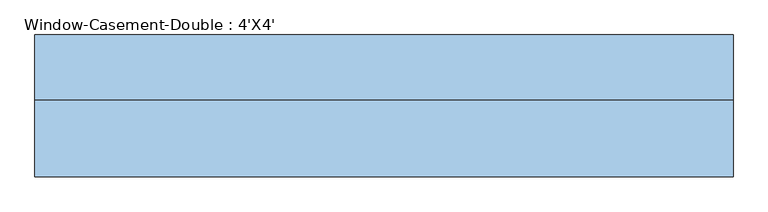
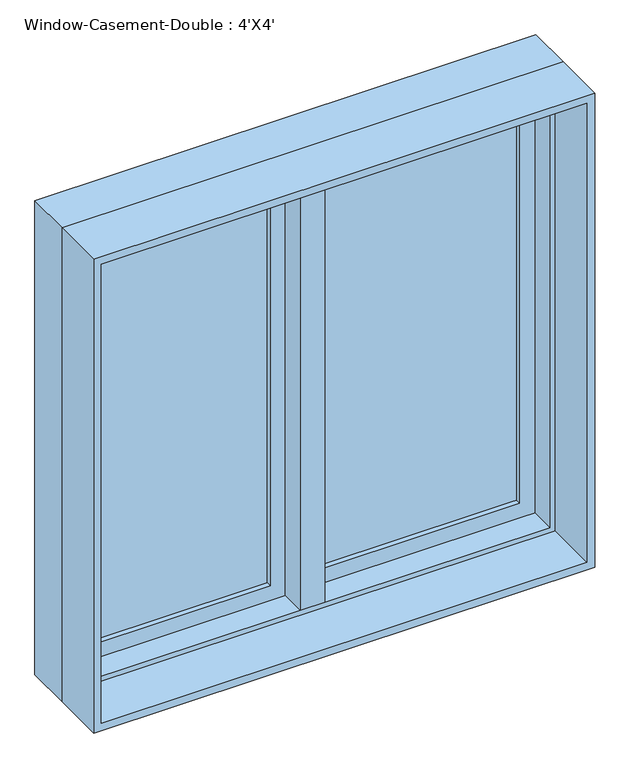
"""IFC4 building model written with IfcOpenShell, lengths in millimetres: window geometry, Window-Casement-Double : 4'X4'."""

from ifc_helpers import new_model, si_unit, frame, origin, place, context, project, spatial, polyline, outline, extrude, faceted_brep, source, transform, mapped, element, save


def window_casement_double_4_x4_af3140d2(model_context):
    return source(origin(), model_context, "Body", "SolidModel", [
        faceted_brep([(9.525, 133.35, 2120.9), (-9.525, 133.35, 2120.9), (-9.525, 82.55, 2120.9), (9.525, 82.55, 2120.9), (9.525, 133.35, 927.1), (9.525, 82.55, 927.1), (-9.525, 82.55, 927.1), (-9.525, 133.35, 927.1), (-9.525, 82.55, 946.15), (-9.525, 82.55, 2101.85), (-30.1625, 82.55, 946.15), (-30.1625, 82.55, 2101.85), (-30.1625, 19.05, 946.15), (-30.1625, 19.05, 2101.85), (30.1625, 19.05, 946.15), (30.1625, 19.05, 2101.85), (30.1625, 82.55, 946.15), (30.1625, 82.55, 2101.85), (9.525, 82.55, 946.15), (9.525, 82.55, 2101.85)], [[[0, 1, 2, 3]], [[4, 5, 6, 7]], [[1, 0, 4, 7]], [[2, 1, 7, 6, 8, 9]], [[9, 8, 10, 11]], [[11, 10, 12, 13]], [[13, 12, 14, 15]], [[15, 14, 16, 17]], [[17, 16, 18, 19]], [[0, 3, 19, 18, 5, 4]], [[18, 8, 6, 5]], [[9, 19, 3, 2]], [[8, 18, 16, 14, 12, 10]], [[19, 9, 11, 13, 15, 17]]]),
        extrude(outline(polyline([(-66.675, 114.3), (-66.675, 107.95), (-539.75, 107.95), (-539.75, 114.3), (-66.675, 114.3)])), frame((0.0, 0.0, 984.25), z_axis=(0.0, 0.0, 1.0), x_axis=(1.0, 0.0, 0.0)), (0.0, 0.0, 1.0), 1079.5),
        extrude(outline(polyline([(-539.75, 95.25), (-539.75, 101.6), (-66.675, 101.6), (-66.675, 95.25), (-539.75, 95.25)])), frame((0.0, 0.0, 984.25), z_axis=(0.0, 0.0, 1.0), x_axis=(1.0, 0.0, 0.0)), (0.0, 0.0, 1.0), 1079.5),
        extrude(outline(polyline([(539.75, 114.3), (539.75, 107.95), (66.675, 107.95), (66.675, 114.3), (539.75, 114.3)])), frame((0.0, 0.0, 984.25), z_axis=(0.0, 0.0, 1.0), x_axis=(1.0, 0.0, 0.0)), (0.0, 0.0, 1.0), 1079.5),
        extrude(outline(polyline([(66.675, 95.25), (66.675, 101.6), (539.75, 101.6), (539.75, 95.25), (66.675, 95.25)])), frame((0.0, 0.0, 984.25), z_axis=(0.0, 0.0, 1.0), x_axis=(1.0, 0.0, 0.0)), (0.0, 0.0, 1.0), 1079.5),
        extrude(outline(polyline([(2120.9, -596.9), (927.1, -596.9), (927.1, -9.525), (2120.9, -9.525), (2120.9, -596.9)]), holes=[polyline([(2063.75, -66.675), (984.25, -66.675), (984.25, -539.75), (2063.75, -539.75), (2063.75, -66.675)])]), frame((0.0, 82.55, 0.0), z_axis=(0.0, 1.0, 0.0), x_axis=(0.0, 0.0, 1.0)), (0.0, 0.0, 1.0), 44.45),
        extrude(outline(polyline([(927.1, 596.9), (2120.9, 596.9), (2120.9, 9.525), (927.1, 9.525), (927.1, 596.9)]), holes=[polyline([(984.25, 66.675), (2063.75, 66.675), (2063.75, 539.75), (984.25, 539.75), (984.25, 66.675)])]), frame((0.0, 82.55, 0.0), z_axis=(0.0, 1.0, 0.0), x_axis=(0.0, 0.0, 1.0)), (0.0, 0.0, 1.0), 44.45),
        extrude(outline(polyline([(2133.6, -609.6), (914.4, -609.6), (914.4, 609.6), (2133.6, 609.6), (2133.6, -609.6)]), holes=[polyline([(2114.55, 590.55), (933.45, 590.55), (933.45, -590.55), (2114.55, -590.55), (2114.55, 590.55)])]), frame((0.0, -114.3, 0.0), z_axis=(0.0, 1.0, 0.0), x_axis=(0.0, 0.0, 1.0)), (0.0, 0.0, 1.0), 133.35),
        faceted_brep([(577.85, 82.55, 2101.85), (577.85, 19.05, 2101.85), (-577.85, 19.05, 2101.85), (-577.85, 82.55, 2101.85), (596.9, 133.35, 2120.9), (596.9, 82.55, 2120.9), (-596.9, 82.55, 2120.9), (-596.9, 133.35, 2120.9), (609.6, 19.05, 2133.6), (609.6, 133.35, 2133.6), (-609.6, 133.35, 2133.6), (-609.6, 19.05, 2133.6), (-577.85, 19.05, 946.15), (-577.85, 82.55, 946.15), (-596.9, 82.55, 927.1), (-596.9, 133.35, 927.1), (-609.6, 133.35, 914.4), (-609.6, 19.05, 914.4), (577.85, 19.05, 946.15), (577.85, 82.55, 946.15), (596.9, 82.55, 927.1), (596.9, 133.35, 927.1), (609.6, 133.35, 914.4), (609.6, 19.05, 914.4)], [[[0, 1, 2, 3]], [[4, 5, 6, 7]], [[8, 9, 10, 11]], [[3, 2, 12, 13]], [[7, 6, 14, 15]], [[11, 10, 16, 17]], [[13, 12, 18, 19]], [[15, 14, 20, 21]], [[17, 16, 22, 23]], [[11, 17, 23, 8], [1, 18, 12, 2]], [[19, 18, 1, 0]], [[5, 20, 14, 6], [3, 13, 19, 0]], [[21, 20, 5, 4]], [[23, 22, 9, 8]], [[9, 22, 16, 10], [7, 15, 21, 4]]]),
    ])


if __name__ == "__main__":
    model = new_model("IFC4")
    model_context = context("Model", 3, world=origin())
    ifc_project = project(units=[si_unit("LENGTHUNIT", "METRE", prefix="MILLI")], contexts=[model_context])
    site = spatial("IfcSite", under=ifc_project)
    building = spatial("IfcBuilding", under=site)
    placement = place(None, origin())
    window_casement_double_4_x4_shape = window_casement_double_4_x4_af3140d2(model_context)
    element("IfcWindow", 1, ObjectType="Window-Casement-Double : 4'X4'", at=placement, inside=building, context=model_context, shape_type="MappedRepresentation", body=[
        mapped(window_casement_double_4_x4_shape, transform((0.0, 0.0, 0.0), x_axis=(1.0, 0.0, 0.0), y_axis=(0.0, 1.0, 0.0), z_axis=(0.0, 0.0, 1.0))),
    ])
    save(model, "model.ifc")

# Revit data of these elements
# Type "Window-Casement-Double : 4'X4'"
#   Type Mark = "19"
#   Fire Rating = "0.5h"
#   Assembly Code = "B2020100"
#   Analytic Construction = "Double glazing - domestic"
#   Frame Extension [instance default] = 0' - 0 1/4"
#   Window Inset [instance default] = 0' - 0"
#   Wall Thickness [instance default] = 0' - 6"
#   Interior Wall Closure [instance default] = 0' - 2 1/4"
#   Half Width = 2' - 0"
#   Visual Light Transmittance = 0.81
#   Thermal Resistance (R) = 1.8146 (h·ft²·°F)/BTU
#   Solar Heat Gain Coefficient = 0.76
#   Rough Width = 4' - 0 1/2"
#   Rough Height = 4' - 0 1/2"
#   Height = 4' - 0"
#   Heat Transfer Coefficient (U) = 0.5511 BTU/(h·ft²·°F)
#   Exterior Wall Closure [instance default] = 0' - 1 1/4"
#   Extension Jamb [instance default] = 0' - 2 1/4"
#   Default Sill Height = 3' - 0"
#   Width = 4' - 0"
#   Muntin Visibility = yes
#   Interior Trim Visibility [instance default] = yes
#   Exterior Trim Visibility [instance default] = yes
#   Extension Jamb Visibility [instance default] = yes
#   Interior Trim Material = Wood - Stained
#   Muntin Pattern = Muntin Pattern_2x2 : Muntin Pattern_2x2
#   Interior Trim = Trim-Window-Interior-Flat : Picture Frame
#   Interior Frame Material = Wood - Stained
#   Glass Panel Material = Glass
#   Exterior Trim Material = Clad - White
#   Exterior Trim = Trim-Window-Exterior-Flat : with Sill
#   Exterior Frame Material = Clad - White
#   Wall Closure = (empty or 0)
# Element 1 (IfcWindow, "Window-Casement-Double : 4'X4'")
#   Wall Thickness = 0' - 9"
#   Extension Jamb = 0' - 5 1/4"
#   Materials on its faces: "Wood - Stained", "Glass", "Clad - White"
# Materials
#   "Wood - Stained": class "Wood", colour RGB 224 178 126, transparency 0, Cost = 0
#   "Glass": class "Glass", colour RGB 0 128 192, transparency 0.75, Description = "Soda Lime Glass", Cost = 0
#   "Clad - White": class "Wood", colour RGB 242 242 238, transparency 0, Cost = 0
